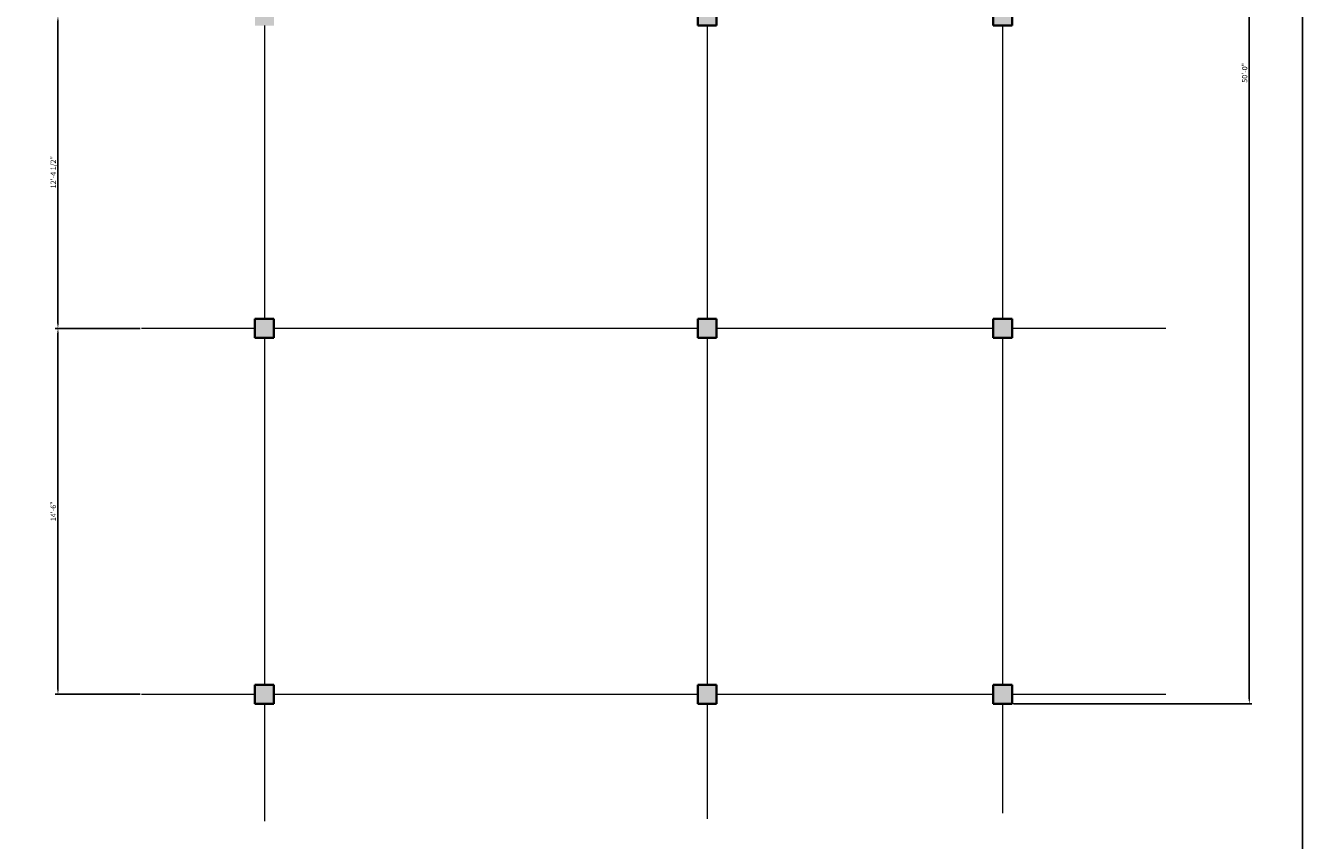
# Model space of a CAD drawing. Units: inches. Extents: x 2169 to 10664, y 1669 to 6352.
# Tile 5 of 17: x 2644 to 3251, y 2091 to 2479. Entities that reach past the tile are written whole.
import ezdxf

# ---------------------------------------------------------------- set-up
doc = ezdxf.new("R2010")
doc.units = ezdxf.units.IN
for name, color, linetype, lineweight in [('A-ANNO-DIMS', 3, 'Continuous', 18), ('A-ANNO-TTLB', 7, 'Continuous', 25), ('A-COLS', 3, 'Continuous', 35), ('A-COLS-PATT', 3, 'Continuous', 13), ('A-GRID', 1, 'Continuous', 13)]:
    doc.layers.add(name, color=color, linetype=linetype, lineweight=lineweight)
doc.styles.get("Standard").update_dxf_attribs({"font": 'arial.ttf'})
doc.dimstyles.new('ISO-25', dxfattribs={"dimtxt": 2.5, "dimasz": 2.5, "dimexe": 1.25, "dimexo": 0.625, "dimtad": 1, "dimdec": 0, "dimlunit": 3, "dimtxsty": 'Standard', "dimcen": 2.5, "dimadec": 0, "dimazin": 0, "dimtfac": 1, "dimtdec": 0, "dimtmove": 0, "dimatfit": 3, "dimfxl": 1, "dimarcsym": 0})

# ---------------------------------------------------------------- blocks, each defined once
blk = doc.blocks.new('COL-9X9')
for p, q in [((0, 9), (9, 9)), ((0, 0), (0, 9)), ((9, 9), (9, 0)), ((9, 0), (0, 0))]:
    blk.add_line(p, q)
blk = doc.blocks.new('*D89')
at = {"layer": 'A-ANNO-DIMS', "color": 0, "lineweight": -2, "transparency": 16777216}
for p, q in [((2698.46, 2483.18), (2658.14, 2483.18)), ((2659.39, 2480.68), (2659.39, 2337.18)), ((2698.46, 2334.68), (2658.14, 2334.68))]:
    blk.add_line(p, q, dxfattribs=at)
at = {"layer": 'A-ANNO-DIMS', "color": 0, "transparency": 16777216}
for points in [[(2658.97, 2480.68), (2659.8, 2480.68), (2659.39, 2483.18)], [(2658.97, 2337.18), (2659.8, 2337.18), (2659.39, 2334.68)]]:
    blk.add_solid(points, dxfattribs=at)
at = {"layer": 'Defpoints', "color": 0, "transparency": 16777216}
for p in [(2699.09, 2483.18), (2659.39, 2334.68), (2699.09, 2334.68)]:
    blk.add_point(p, dxfattribs=at)
at = {"layer": 'A-ANNO-DIMS', "color": 0, "transparency": 16777216, "insert": (2657.47, 2408.93), "char_height": 2.5, "attachment_point": 5, "rotation": 90}
blk.add_mtext('12\'-4 1/2"', dxfattribs=at)
blk = doc.blocks.new('*D90')
at = {"layer": 'A-ANNO-DIMS', "color": 0, "lineweight": -2, "transparency": 16777216}
for p, q in [((2698.46, 2334.68), (2658.14, 2334.68)), ((2659.39, 2332.18), (2659.39, 2163.18)), ((2698.46, 2160.68), (2658.14, 2160.68))]:
    blk.add_line(p, q, dxfattribs=at)
at = {"layer": 'A-ANNO-DIMS', "color": 0, "transparency": 16777216}
for points in [[(2658.97, 2332.18), (2659.8, 2332.18), (2659.39, 2334.68)], [(2658.97, 2163.18), (2659.8, 2163.18), (2659.39, 2160.68)]]:
    blk.add_solid(points, dxfattribs=at)
at = {"layer": 'Defpoints', "color": 0, "transparency": 16777216}
for p in [(2699.09, 2334.68), (2659.39, 2160.68), (2699.09, 2160.68)]:
    blk.add_point(p, dxfattribs=at)
at = {"layer": 'A-ANNO-DIMS', "color": 0, "transparency": 16777216, "insert": (2657.49, 2247.68), "char_height": 2.5, "attachment_point": 5, "rotation": 90}
blk.add_mtext('14\'-6"', dxfattribs=at)
blk = doc.blocks.new('*D92')
at = {"layer": 'A-ANNO-DIMS', "color": 0, "lineweight": -2, "transparency": 16777216}
for p, q in [((3113.7, 2756.18), (3227.1, 2756.18)), ((3225.85, 2753.68), (3225.85, 2158.68)), ((3113.7, 2156.18), (3227.1, 2156.18))]:
    blk.add_line(p, q, dxfattribs=at)
at = {"layer": 'A-ANNO-DIMS', "color": 0, "transparency": 16777216}
for points in [[(3225.43, 2753.68), (3226.27, 2753.68), (3225.85, 2756.18)], [(3225.43, 2158.68), (3226.27, 2158.68), (3225.85, 2156.18)]]:
    blk.add_solid(points, dxfattribs=at)
at = {"layer": 'Defpoints', "color": 0, "transparency": 16777216}
for p in [(3113.07, 2756.18), (3113.07, 2156.18), (3225.85, 2156.18)]:
    blk.add_point(p, dxfattribs=at)
at = {"layer": 'A-ANNO-DIMS', "color": 0, "transparency": 16777216, "insert": (3223.95, 2456.18), "char_height": 2.5, "attachment_point": 5, "rotation": 90}
blk.add_mtext('50\'-0"', dxfattribs=at)

msp = doc.modelspace()

# ---------------------------------------------------------------- hatches: boundary and pattern name
at = {"layer": 'A-COLS-PATT'}
h = msp.add_hatch(color=256, dxfattribs=at)
h.dxf.hatch_style = 1
h.paths.add_polyline_path([(2762.07, 2165.18), (2753.07, 2165.18), (2753.07, 2156.18), (2762.07, 2156.18)])
h.paths.add_polyline_path([(2972.57, 2165.18), (2963.57, 2165.18), (2963.57, 2156.18), (2972.57, 2156.18)])
h.paths.add_polyline_path([(3113.07, 2165.18), (3104.07, 2165.18), (3104.07, 2156.18), (3113.07, 2156.18)])
h.paths.add_polyline_path([(3113.07, 2330.18), (3113.07, 2339.18), (3104.07, 2339.18), (3104.07, 2330.18)])
h.paths.add_polyline_path([(2972.57, 2339.18), (2963.57, 2339.18), (2963.57, 2330.18), (2972.57, 2330.18)])
h.paths.add_polyline_path([(2762.07, 2330.18), (2762.07, 2339.18), (2753.07, 2339.18), (2753.07, 2330.18)])
h.paths.add_polyline_path([(2753.07, 2478.68), (2762.07, 2478.68), (2762.07, 2487.68), (2753.07, 2487.68)])
h.paths.add_polyline_path([(2963.57, 2487.68), (2963.57, 2478.68), (2972.57, 2478.68), (2972.57, 2487.68)])
h.paths.add_polyline_path([(3104.07, 2487.68), (3104.07, 2478.68), (3113.07, 2478.68), (3113.07, 2487.68)])
h.paths.add_polyline_path([(3104.07, 2602.68), (3113.07, 2602.68), (3113.07, 2611.68), (3104.07, 2611.68)])
h.paths.add_polyline_path([(2963.57, 2602.68), (2972.57, 2602.68), (2972.57, 2611.68), (2963.57, 2611.68)])
h.paths.add_polyline_path([(2753.07, 2611.68), (2753.07, 2602.68), (2762.07, 2602.68), (2762.07, 2611.68)])
h.paths.add_polyline_path([(2762.07, 2747.18), (2762.07, 2756.18), (2753.07, 2756.18), (2753.07, 2747.18)])
h.paths.add_polyline_path([(2972.57, 2747.18), (2972.57, 2756.18), (2963.57, 2756.18), (2963.57, 2747.18)])
h.paths.add_polyline_path([(3104.07, 2756.18), (3104.07, 2747.18), (3113.07, 2747.18), (3113.07, 2756.18)])

# ---------------------------------------------------------------- linework, layer by layer
at = {"layer": 'A-ANNO-TTLB'}
msp.add_lwpolyline([(2169.45, 2838.28), (3251.13, 2838.28), (3251.13, 1669.34), (2169.45, 1669.34)], close=True, dxfattribs=at)
at = {"layer": 'A-COLS'}
msp.add_line((3104.07, 2330.18), (3104.07, 2339.18), dxfattribs=at)
at = {"layer": 'A-GRID'}
for p, q in [((2757.57, 2478.68), (2757.57, 2339.18)), ((2968.07, 2478.68), (2968.07, 2339.18)), ((3108.57, 2478.68), (3108.57, 2339.18)), ((2753.07, 2334.68), (2699.09, 2334.68)), ((2963.57, 2334.68), (2762.07, 2334.68)), ((3104.07, 2334.68), (2972.57, 2334.68)), ((3186.15, 2334.68), (3113.07, 2334.68)), ((2757.57, 2330.18), (2757.57, 2165.18)), ((2968.07, 2330.18), (2968.07, 2165.18)), ((3108.57, 2330.18), (3108.57, 2165.18)), ((2699.09, 2160.68), (2753.07, 2160.68)), ((2757.57, 2156.18), (2757.57, 2100.37)), ((2762.07, 2160.68), (2963.57, 2160.68)), ((2968.07, 2156.18), (2968.07, 2101.51)), ((2972.57, 2160.68), (3104.07, 2160.68)), ((3108.57, 2156.18), (3108.57, 2104.13)), ((3113.07, 2160.68), (3186.15, 2160.68))]:
    msp.add_line(p, q, dxfattribs=at)

# ---------------------------------------------------------------- block references
at = {"layer": 'A-COLS', "rotation": 180}
for p in [(2972.57, 2487.68), (3113.07, 2487.68), (2762.07, 2339.18), (2972.57, 2339.18), (3113.07, 2339.18), (2762.07, 2165.18), (2972.57, 2165.18), (3113.07, 2165.18)]:
    msp.add_blockref('COL-9X9', p, dxfattribs=at)

# ---------------------------------------------------------------- dimensions: what is measured, and where the dimension line sits
at = {"layer": 'A-ANNO-DIMS'}
for base, p1, p2, picture, middle in [((3225.85, 2156.18), (3113.07, 2756.18), (3113.07, 2156.18), '*D92', (3223.95, 2456.18)), ((2659.39, 2334.68), (2699.09, 2483.18), (2699.09, 2334.68), '*D89', (2657.47, 2408.93)), ((2659.39, 2160.68), (2699.09, 2334.68), (2699.09, 2160.68), '*D90', (2657.49, 2247.68))]:
    dim = msp.add_linear_dim(base=base, p1=p1, p2=p2, angle=90, dimstyle='ISO-25', override={"dimdec": 1, "dimlfac": 1, "dimrnd": 0, "dimzin": 1, "dimdsep": 46, "dimlunit": 4, "dimfrac": 2}, dxfattribs=at)
    dim.commit()
    dim.dimension.update_dxf_attribs({"geometry": picture, "text_midpoint": middle})

doc.saveas('drawing.dxf')
